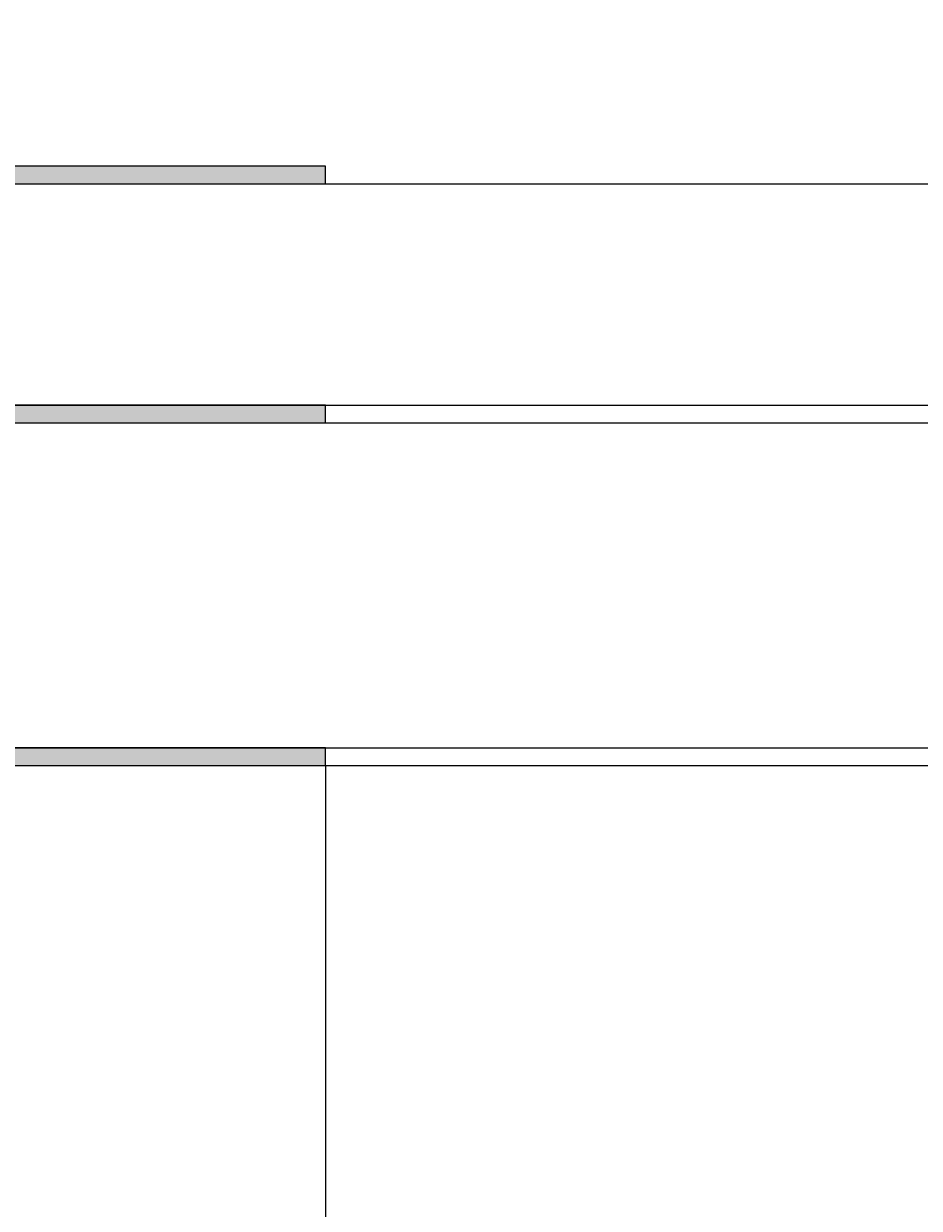
# Model space of a CAD drawing. Units: inches. Extents: x 35362 to 73946, y 43607 to 67532.
# Tile 133 of 134: x 69530 to 70544, y 44948 to 46290. Entities that reach past the tile are written whole.
import ezdxf

# ---------------------------------------------------------------- set-up
doc = ezdxf.new("R2010")
doc.units = ezdxf.units.IN
doc.header["$MEASUREMENT"] = 0
for name, color, linetype, lineweight in [('A-ANNO-DIMS', 2, 'Continuous', 18), ('E-SYMB', 1, 'Continuous', 25), ('E-SYMB-PATT', 1, 'Continuous', 13)]:
    doc.layers.add(name, color=color, linetype=linetype, lineweight=lineweight)
doc.styles.get("Standard").update_dxf_attribs({"font": 'arial.ttf'})
doc.dimstyles.get("Standard").update_dxf_attribs({"dimtxt": 0.18, "dimasz": 0.18, "dimexe": 0.18, "dimexo": 0.0625, "dimgap": 0.09, "dimtad": 0, "dimtih": 1, "dimtoh": 1, "dimdec": 4, "dimzin": 0, "dimdsep": 46, "dimtxsty": 'Standard', "dimcen": 0.09, "dimadec": 0, "dimazin": 0, "dimtfac": 1, "dimtdec": 4, "dimtofl": 0, "dimtmove": 0, "dimatfit": 3, "dimfxl": 1, "dimtolj": 1, "dimtzin": 0, "dimarcsym": 0})

# ---------------------------------------------------------------- blocks, each defined once
blk = doc.blocks.new('CT-CORE')
for p, q in [((-0.0004610742907971, 1387.996120092102), (-0.0004610742907971, -5.34733626409e-05)), ((19.99953892572375, 1387.996120092102), (-0.0004610742907971, 1387.996120092102)), ((19.9995389257092, -5.34733626409e-05), (19.99953892572375, 1387.996120092102)), ((270.6681283192447, 1387.996120092102), (270.6681283192447, -5.34733626409e-05)), ((290.6681283192593, 1387.996120092102), (270.6681283192447, 1387.996120092102)), ((290.6681283192447, -5.34733626409e-05), (290.6681283192593, 1387.996120092102)), ((658.9826659540267, 1387.996120092102), (658.9826659540267, 1014.585417332389)), ((678.9826659540413, 1387.996120092102), (658.9826659540267, 1387.996120092102)), ((678.9826659540413, 1015.434583844784), (678.9826659540413, 1387.996120092102)), ((658.9826659540267, 544.3844491987692), (658.9826659540267, -5.34733626409e-05)), ((678.9826659540267, -5.34733626409e-05), (678.9826659540413, 543.5352826863744)), ((-0.0004610742907971, -5.34733626409e-05), (19.9995389257092, -5.34733626409e-05)), ((270.6681283192447, -5.34733626409e-05), (290.6681283192447, -5.34733626409e-05)), ((658.9826659540267, -5.34733626409e-05), (678.9826659540267, -5.34733626409e-05))]:
    blk.add_line(p, q)
blk.add_arc((678.9826659540267, 779.4849332655793), 235.9496505792049, 90, 270)
blk = doc.blocks.new('*D5')
at = {"layer": 'A-ANNO-DIMS', "color": 0, "lineweight": -2, "transparency": 16777216}
for p, q in [((37121.949085, 46919.318283), (37121.949085, 43606.678996)), ((69871.496302, 45449.831951), (69871.496302, 43606.678996)), ((37122.129085, 43606.858996), (53496.2943647142, 43606.858996)), ((69871.316302, 43606.858996), (53497.15102228581, 43606.858996))]:
    blk.add_line(p, q, dxfattribs=at)
at = {"layer": 'A-ANNO-DIMS', "color": 0, "transparency": 16777216}
for points in [[(37122.129085, 43606.888996), (37122.129085, 43606.828996), (37121.949085, 43606.858996)], [(69871.316302, 43606.888996), (69871.316302, 43606.828996), (69871.496302, 43606.858996)]]:
    blk.add_solid(points, dxfattribs=at)
at = {"layer": 'Defpoints', "color": 0, "transparency": 16777216}
for p in [(37121.949085, 46919.380783), (69871.496302, 45449.894451), (69871.496302, 43606.858996)]:
    blk.add_point(p, dxfattribs=at)
at = {"layer": 'A-ANNO-DIMS', "color": 0, "transparency": 16777216, "insert": (53496.7226935, 43606.858996), "char_height": 0.18, "attachment_point": 5}
blk.add_mtext('\\A1;32750', dxfattribs=at)
blk = doc.blocks.new('*D6')
at = {"layer": 'A-ANNO-DIMS', "color": 0, "lineweight": -2, "transparency": 16777216}
for p, q in [((72185.645666, 53702.123839), (72185.645666, 43606.678996)), ((69871.496302, 45449.831951), (69871.496302, 43606.678996)), ((69871.67630199999, 43606.858996), (71028.21104539152, 43606.858996)), ((72185.465666, 43606.858996), (71028.93092260844, 43606.858996))]:
    blk.add_line(p, q, dxfattribs=at)
at = {"layer": 'A-ANNO-DIMS', "color": 0, "transparency": 16777216}
for points in [[(69871.67630199999, 43606.888996), (69871.67630199999, 43606.828996), (69871.496302, 43606.858996)], [(72185.465666, 43606.888996), (72185.465666, 43606.828996), (72185.645666, 43606.858996)]]:
    blk.add_solid(points, dxfattribs=at)
at = {"layer": 'Defpoints', "color": 0, "transparency": 16777216}
for p in [(72185.645666, 53702.186339), (69871.496302, 45449.894451), (72185.645666, 43606.858996)]:
    blk.add_point(p, dxfattribs=at)
at = {"layer": 'A-ANNO-DIMS', "color": 0, "transparency": 16777216, "insert": (71028.57098399999, 43606.858996), "char_height": 0.18, "attachment_point": 5}
blk.add_mtext('\\A1;2314', dxfattribs=at)
blk = doc.blocks.new('*D7')
at = {"layer": 'A-ANNO-DIMS', "color": 0, "lineweight": -2, "transparency": 16777216}
for p, q in [((72185.70816600003, 53702.18633900003), (73945.82566600003, 53702.18633900003)), ((73945.64566600005, 53702.00633900003), (73945.64566600005, 49576.22229813781)), ((73945.64566600005, 45450.07445100001), (73945.64566600005, 49575.85849186223)), ((69871.55880200003, 45449.89445100001), (73945.82566600003, 45449.89445100001))]:
    blk.add_line(p, q, dxfattribs=at)
at = {"layer": 'A-ANNO-DIMS', "color": 0, "transparency": 16777216}
for points in [[(73945.61566600006, 53702.00633900003), (73945.67566600005, 53702.00633900003), (73945.64566600005, 53702.18633900003)], [(73945.61566600006, 45450.07445100001), (73945.67566600005, 45450.07445100001), (73945.64566600005, 45449.89445100001)]]:
    blk.add_solid(points, dxfattribs=at)
at = {"layer": 'Defpoints', "color": 0, "transparency": 16777216}
for p in [(72185.64566600003, 53702.18633900003), (73945.64566600005, 53702.18633900003), (69871.49630200001, 45449.89445100001)]:
    blk.add_point(p, dxfattribs=at)
at = {"layer": 'A-ANNO-DIMS', "color": 0, "transparency": 16777216, "insert": (73945.64566600005, 49576.04039499998), "char_height": 0.18, "attachment_point": 5}
blk.add_mtext('\\A1;8252', dxfattribs=at)
blk = doc.blocks.new('*D74')
at = {"layer": 'A-ANNO-DIMS', "color": 0, "lineweight": -2, "transparency": 16777216}
for p, q in [((55181.69646300003, 46108.87757800001), (73945.82566600003, 46108.87757800001)), ((73945.64566600005, 46108.69757800001), (73945.64566600005, 45983.7251866378)), ((73945.64566600005, 45858.38898900001), (73945.64566600005, 45983.36138036223)), ((55181.69646300003, 45858.20898900001), (73945.82566600003, 45858.20898900001))]:
    blk.add_line(p, q, dxfattribs=at)
at = {"layer": 'A-ANNO-DIMS', "color": 0, "transparency": 16777216}
for points in [[(73945.61566600006, 46108.69757800001), (73945.67566600005, 46108.69757800001), (73945.64566600005, 46108.87757800001)], [(73945.61566600006, 45858.38898900001), (73945.67566600005, 45858.38898900001), (73945.64566600005, 45858.20898900001)]]:
    blk.add_solid(points, dxfattribs=at)
at = {"layer": 'Defpoints', "color": 0, "transparency": 16777216}
for p in [(55181.63396300002, 46108.87757800001), (55181.63396300002, 45858.20898900001), (73945.64566600005, 45858.20898900001)]:
    blk.add_point(p, dxfattribs=at)
at = {"layer": 'A-ANNO-DIMS', "color": 0, "transparency": 16777216, "insert": (73945.64566600005, 45983.54328349999), "char_height": 0.18, "attachment_point": 5}
blk.add_mtext('\\A1;250.67', dxfattribs=at)
blk = doc.blocks.new('*D75')
at = {"layer": 'A-ANNO-DIMS', "color": 0, "lineweight": -2, "transparency": 16777216}
for p, q in [((55181.69646300003, 45838.20898900001), (73945.82566600003, 45838.20898900001)), ((73945.64566600005, 45838.02898900001), (73945.64566600005, 45654.23368452933)), ((73945.64566600005, 45470.07445100001), (73945.64566600005, 45653.86975547068)), ((55181.69646300003, 45469.89445100001), (73945.82566600003, 45469.89445100001))]:
    blk.add_line(p, q, dxfattribs=at)
at = {"layer": 'A-ANNO-DIMS', "color": 0, "transparency": 16777216}
for points in [[(73945.61566600006, 45838.02898900001), (73945.67566600005, 45838.02898900001), (73945.64566600005, 45838.20898900001)], [(73945.61566600006, 45470.07445100001), (73945.67566600005, 45470.07445100001), (73945.64566600005, 45469.89445100001)]]:
    blk.add_solid(points, dxfattribs=at)
at = {"layer": 'Defpoints', "color": 0, "transparency": 16777216}
for p in [(55181.63396300002, 45838.20898900001), (55181.63396300002, 45469.89445100001), (73945.64566600005, 45469.89445100001)]:
    blk.add_point(p, dxfattribs=at)
at = {"layer": 'A-ANNO-DIMS', "color": 0, "transparency": 16777216, "insert": (73945.64566600005, 45654.05171999998), "char_height": 0.18, "attachment_point": 5}
blk.add_mtext('\\A1;368.3', dxfattribs=at)

msp = doc.modelspace()

# ---------------------------------------------------------------- hatches: boundary and pattern name
at = {"layer": 'E-SYMB-PATT'}
h = msp.add_hatch(color=256, dxfattribs=at)
h.dxf.hatch_style = 1
h.paths.add_polyline_path([(69871.49630189747, 46108.87757831767), (69871.49630189747, 46128.87757831768), (68483.50012833202, 46128.87757831768), (68483.50012833202, 46108.87757831768)])
h = msp.add_hatch(color=256, dxfattribs=at)
h.dxf.hatch_style = 1
h.paths.add_polyline_path([(69871.49630189747, 45838.20898892413), (69871.49630189747, 45858.20898892414), (68483.50012833202, 45858.20898892414), (68483.50012833202, 45838.20898892414)])
h = msp.add_hatch(color=256, dxfattribs=at)
h.dxf.hatch_style = 1
h.paths.add_polyline_path([(69027.03546449174, 45449.89445128935, -0.0212196039209565), (69027.88463100414, 45469.89445128936), (69011.01171653513, 45469.89445128936, 0.0200709024740955), (69010.20855689044, 45449.89445128935)])
h.paths.add_polyline_path([(69010.20855689044, 45449.89445128935, -0.0200709024740953), (69011.01171653513, 45469.89445128936), (68483.50012833202, 45469.89445128936), (68483.50012833202, 45449.89445128936)])
h.paths.add_polyline_path([(69871.49630189747, 45449.89445128935), (69871.49630189747, 45469.89445128936), (69508.24154776601, 45469.89445128936, -0.0200709024740959), (69509.04470741072, 45449.89445128935)])
h.paths.add_polyline_path([(69509.04470741072, 45449.89445128935, 0.020070902474096), (69508.24154776601, 45469.89445128936), (69498.08559913776, 45469.89445128936, -0.0212196039209564), (69498.93476565015, 45449.89445128935)])

# ---------------------------------------------------------------- block references
at = {"layer": 'E-SYMB', "rotation": 269.9999999999974}
msp.add_blockref('CT-CORE', (68483.50018180539, 46128.87711724339), dxfattribs=at)

# ---------------------------------------------------------------- dimensions: what is measured, and where the dimension line sits
at = {"layer": 'A-ANNO-DIMS'}
for base, p1, p2, picture, middle in [((72185.645666, 43606.858996), (69871.496302, 45449.894451), (72185.645666, 53702.186339), '*D6', (71028.57098399999, 43606.858996)), ((69871.496302, 43606.858996), (37121.949085, 46919.380783), (69871.496302, 45449.894451), '*D5', (53496.7226935, 43606.858996))]:
    dim = msp.add_linear_dim(base=base, p1=p1, p2=p2, dimstyle='Standard', override={"dimdec": 0, "dimlfac": 1, "dimrnd": 0, "dimzin": 0, "dimdsep": 46, "dimlunit": 2}, dxfattribs=at)
    dim.commit()
    dim.dimension.update_dxf_attribs({"geometry": picture, "text_midpoint": middle})
for base, p1, p2, override, picture, middle in [((73945.64566600005, 53702.18633900003), (69871.496302, 45449.894451), (72185.645666, 53702.186339), {"dimdec": 0, "dimlfac": 1, "dimrnd": 0, "dimzin": 0, "dimdsep": 46, "dimlunit": 2}, '*D7', (73945.64566600005, 49576.04039499998)), ((73945.64566600005, 45858.20898900001), (55181.633963, 46108.877578), (55181.633963, 45858.20898899999), {"dimdec": 2, "dimlfac": 1, "dimrnd": 0, "dimzin": 0, "dimdsep": 46, "dimlunit": 2}, '*D74', (73945.64566600005, 45983.54328349999)), ((73945.64566600005, 45469.89445100001), (55181.633963, 45838.20898899999), (55181.633963, 45469.894451), {"dimdec": 1, "dimlfac": 1, "dimrnd": 0, "dimzin": 0, "dimdsep": 46, "dimlunit": 2}, '*D75', (73945.64566600005, 45654.05171999998))]:
    dim = msp.add_linear_dim(base=base, p1=p1, p2=p2, angle=90, dimstyle='Standard', override=override, dxfattribs=at)
    dim.commit()
    dim.dimension.update_dxf_attribs({"geometry": picture, "text_midpoint": middle})

doc.saveas('drawing.dxf')
